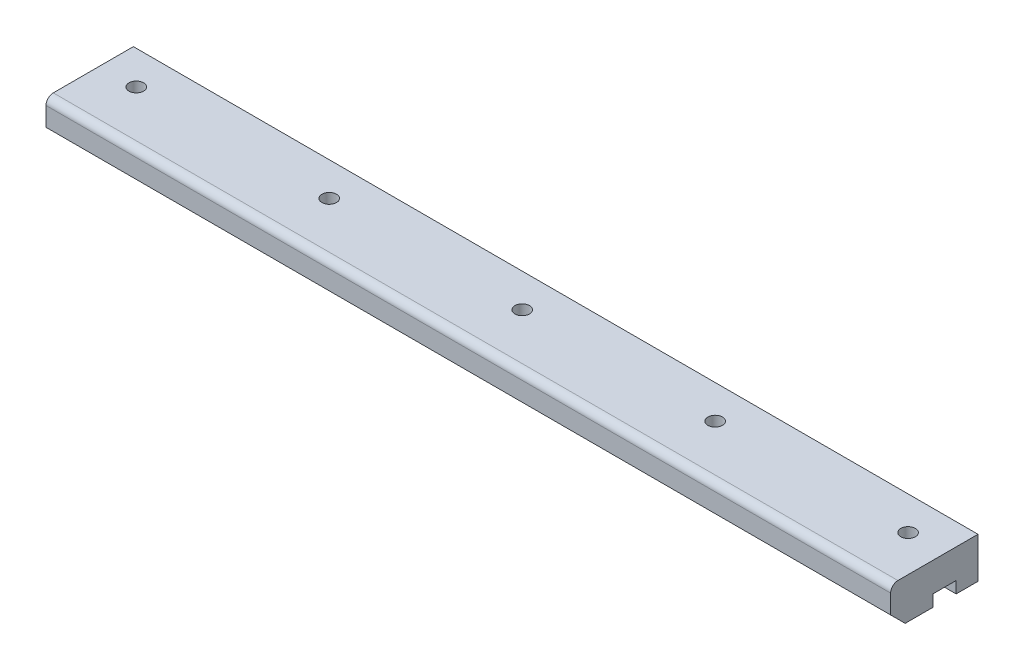
ISO-10303-21;
HEADER;
FILE_DESCRIPTION(('STEP AP214'),'2;1');
FILE_NAME('part.step','',(''),(''),'','','');
FILE_SCHEMA(('AUTOMOTIVE_DESIGN { 1 0 10303 214 1 1 1 1 }'));
ENDSEC;
DATA;
#1=APPLICATION_CONTEXT('core data for automotive mechanical design processes');
#2=APPLICATION_PROTOCOL_DEFINITION('international standard','automotive_design',2000,#1);
#3=PRODUCT_CONTEXT('',#1,'mechanical');
#4=PRODUCT('Part','Part','',(#3));
#5=PRODUCT_RELATED_PRODUCT_CATEGORY('part','',(#4));
#6=PRODUCT_DEFINITION_FORMATION('','',#4);
#7=PRODUCT_DEFINITION_CONTEXT('part definition',#1,'design');
#8=PRODUCT_DEFINITION('design','',#6,#7);
#9=PRODUCT_DEFINITION_SHAPE('','',#8);
#10=(LENGTH_UNIT() NAMED_UNIT(*) SI_UNIT(.MILLI.,.METRE.));
#11=(NAMED_UNIT(*) PLANE_ANGLE_UNIT() SI_UNIT($,.RADIAN.));
#12=(NAMED_UNIT(*) SI_UNIT($,.STERADIAN.) SOLID_ANGLE_UNIT());
#13=UNCERTAINTY_MEASURE_WITH_UNIT(LENGTH_MEASURE(1.E-05),#10,'distance_accuracy_value','');
#14=(GEOMETRIC_REPRESENTATION_CONTEXT(3) GLOBAL_UNCERTAINTY_ASSIGNED_CONTEXT((#13)) GLOBAL_UNIT_ASSIGNED_CONTEXT((#10,
#11,#12)) REPRESENTATION_CONTEXT('',''));
#15=CARTESIAN_POINT('',(0.,0.,0.));
#16=DIRECTION('',(0.,0.,1.));
#17=DIRECTION('',(1.,0.,0.));
#18=AXIS2_PLACEMENT_3D('',#15,#16,#17);
#19=CARTESIAN_POINT('',(580.,28.,-30.));
#20=DIRECTION('',(0.,0.,1.));
#21=DIRECTION('',(1.,0.,0.));
#22=AXIS2_PLACEMENT_3D('',#19,#20,#21);
#23=PLANE('',#22);
#24=DIRECTION('',(0.,1.,0.));
#25=VECTOR('',#24,1.);
#26=CARTESIAN_POINT('',(0.,28.,-30.));
#27=LINE('',#26,#25);
#28=CARTESIAN_POINT('',(0.,0.,-30.));
#29=VERTEX_POINT('',#28);
#30=CARTESIAN_POINT('',(0.,28.,-30.));
#31=VERTEX_POINT('',#30);
#32=EDGE_CURVE('E149',#29,#31,#27,.T.);
#33=ORIENTED_EDGE('',*,*,#32,.T.);
#34=DIRECTION('',(-1.,0.,0.));
#35=VECTOR('',#34,1.);
#36=CARTESIAN_POINT('',(580.,28.,-30.));
#37=LINE('',#36,#35);
#38=CARTESIAN_POINT('',(580.,28.,-30.));
#39=VERTEX_POINT('',#38);
#40=EDGE_CURVE('E11',#39,#31,#37,.T.);
#41=ORIENTED_EDGE('',*,*,#40,.F.);
#42=DIRECTION('',(0.,1.,0.));
#43=VECTOR('',#42,1.);
#44=CARTESIAN_POINT('',(580.,28.,-30.));
#45=LINE('',#44,#43);
#46=CARTESIAN_POINT('',(580.,0.,-30.));
#47=VERTEX_POINT('',#46);
#48=EDGE_CURVE('E170',#47,#39,#45,.T.);
#49=ORIENTED_EDGE('',*,*,#48,.F.);
#50=DIRECTION('',(-1.,0.,0.));
#51=VECTOR('',#50,1.);
#52=CARTESIAN_POINT('',(580.,0.,-30.));
#53=LINE('',#52,#51);
#54=EDGE_CURVE('E144',#47,#29,#53,.T.);
#55=ORIENTED_EDGE('',*,*,#54,.T.);
#56=EDGE_LOOP('',(#33,#41,#49,#55));
#57=FACE_BOUND('',#56,.T.);
#58=ADVANCED_FACE('F39',(#57),#23,.F.);
#59=CARTESIAN_POINT('',(580.,28.,25.));
#60=DIRECTION('',(0.,-1.,0.));
#61=DIRECTION('',(0.,0.,-1.));
#62=AXIS2_PLACEMENT_3D('',#59,#60,#61);
#63=PLANE('',#62);
#64=CARTESIAN_POINT('',(25.,28.,-7.));
#65=DIRECTION('',(0.,1.,0.));
#66=DIRECTION('',(0.,0.,1.));
#67=AXIS2_PLACEMENT_3D('',#64,#65,#66);
#68=CIRCLE('',#67,5.);
#69=CARTESIAN_POINT('',(25.,28.,-1.99999999999999));
#70=VERTEX_POINT('',#69);
#71=EDGE_CURVE('E188',#70,#70,#68,.T.);
#72=ORIENTED_EDGE('',*,*,#71,.F.);
#73=EDGE_LOOP('',(#72));
#74=FACE_BOUND('',#73,.T.);
#75=CARTESIAN_POINT('',(157.5,28.,-7.));
#76=DIRECTION('',(0.,1.,0.));
#77=DIRECTION('',(0.,0.,1.));
#78=AXIS2_PLACEMENT_3D('',#75,#76,#77);
#79=CIRCLE('',#78,4.99999999999999);
#80=CARTESIAN_POINT('',(157.5,28.,-2.00000000000001));
#81=VERTEX_POINT('',#80);
#82=EDGE_CURVE('E306',#81,#81,#79,.T.);
#83=ORIENTED_EDGE('',*,*,#82,.F.);
#84=EDGE_LOOP('',(#83));
#85=FACE_BOUND('',#84,.T.);
#86=CARTESIAN_POINT('',(290.,28.,-7.));
#87=DIRECTION('',(0.,1.,0.));
#88=DIRECTION('',(0.,0.,1.));
#89=AXIS2_PLACEMENT_3D('',#86,#87,#88);
#90=CIRCLE('',#89,4.99999999999999);
#91=CARTESIAN_POINT('',(290.,28.,-2.00000000000001));
#92=VERTEX_POINT('',#91);
#93=EDGE_CURVE('E300',#92,#92,#90,.T.);
#94=ORIENTED_EDGE('',*,*,#93,.F.);
#95=EDGE_LOOP('',(#94));
#96=FACE_BOUND('',#95,.T.);
#97=CARTESIAN_POINT('',(422.5,28.,-7.));
#98=DIRECTION('',(0.,1.,0.));
#99=DIRECTION('',(0.,0.,1.));
#100=AXIS2_PLACEMENT_3D('',#97,#98,#99);
#101=CIRCLE('',#100,4.99999999999999);
#102=CARTESIAN_POINT('',(422.5,28.,-2.00000000000001));
#103=VERTEX_POINT('',#102);
#104=EDGE_CURVE('E310',#103,#103,#101,.T.);
#105=ORIENTED_EDGE('',*,*,#104,.F.);
#106=EDGE_LOOP('',(#105));
#107=FACE_BOUND('',#106,.T.);
#108=CARTESIAN_POINT('',(555.,28.,-7.));
#109=DIRECTION('',(0.,1.,0.));
#110=DIRECTION('',(0.,0.,1.));
#111=AXIS2_PLACEMENT_3D('',#108,#109,#110);
#112=CIRCLE('',#111,5.00000000000004);
#113=CARTESIAN_POINT('',(555.,28.,-1.99999999999995));
#114=VERTEX_POINT('',#113);
#115=EDGE_CURVE('E314',#114,#114,#112,.T.);
#116=ORIENTED_EDGE('',*,*,#115,.F.);
#117=EDGE_LOOP('',(#116));
#118=FACE_BOUND('',#117,.T.);
#119=DIRECTION('',(0.,0.,1.));
#120=VECTOR('',#119,1.);
#121=CARTESIAN_POINT('',(0.,28.,25.));
#122=LINE('',#121,#120);
#123=CARTESIAN_POINT('',(0.,28.,25.));
#124=VERTEX_POINT('',#123);
#125=EDGE_CURVE('E155',#31,#124,#122,.T.);
#126=ORIENTED_EDGE('',*,*,#125,.T.);
#127=DIRECTION('',(-1.,0.,0.));
#128=VECTOR('',#127,1.);
#129=CARTESIAN_POINT('',(580.,28.,25.));
#130=LINE('',#129,#128);
#131=CARTESIAN_POINT('',(580.,28.,25.));
#132=VERTEX_POINT('',#131);
#133=EDGE_CURVE('E48',#132,#124,#130,.T.);
#134=ORIENTED_EDGE('',*,*,#133,.F.);
#135=DIRECTION('',(0.,0.,1.));
#136=VECTOR('',#135,1.);
#137=CARTESIAN_POINT('',(580.,28.,25.));
#138=LINE('',#137,#136);
#139=EDGE_CURVE('E106',#39,#132,#138,.T.);
#140=ORIENTED_EDGE('',*,*,#139,.F.);
#141=ORIENTED_EDGE('',*,*,#40,.T.);
#142=EDGE_LOOP('',(#126,#134,#140,#141));
#143=FACE_BOUND('',#142,.T.);
#144=ADVANCED_FACE('F214',(#74,#85,#96,#107,#118,#143),#63,.F.);
#145=CARTESIAN_POINT('',(580.,23.,25.));
#146=DIRECTION('',(-1.,0.,0.));
#147=DIRECTION('',(0.,0.,1.));
#148=AXIS2_PLACEMENT_3D('',#145,#146,#147);
#149=CYLINDRICAL_SURFACE('',#148,5.);
#150=CARTESIAN_POINT('',(0.,23.,25.));
#151=DIRECTION('',(1.,0.,0.));
#152=DIRECTION('',(0.,0.,-1.));
#153=AXIS2_PLACEMENT_3D('',#150,#151,#152);
#154=CIRCLE('',#153,5.);
#155=CARTESIAN_POINT('',(0.,23.,30.));
#156=VERTEX_POINT('',#155);
#157=EDGE_CURVE('E152',#124,#156,#154,.T.);
#158=ORIENTED_EDGE('',*,*,#157,.T.);
#159=DIRECTION('',(-1.,0.,0.));
#160=VECTOR('',#159,1.);
#161=CARTESIAN_POINT('',(580.,23.,30.));
#162=LINE('',#161,#160);
#163=CARTESIAN_POINT('',(580.,23.,30.));
#164=VERTEX_POINT('',#163);
#165=EDGE_CURVE('E176',#164,#156,#162,.T.);
#166=ORIENTED_EDGE('',*,*,#165,.F.);
#167=CARTESIAN_POINT('',(580.,23.,25.));
#168=DIRECTION('',(1.,0.,0.));
#169=DIRECTION('',(0.,0.,-1.));
#170=AXIS2_PLACEMENT_3D('',#167,#168,#169);
#171=CIRCLE('',#170,5.);
#172=EDGE_CURVE('E233',#132,#164,#171,.T.);
#173=ORIENTED_EDGE('',*,*,#172,.F.);
#174=ORIENTED_EDGE('',*,*,#133,.T.);
#175=EDGE_LOOP('',(#158,#166,#173,#174));
#176=FACE_BOUND('',#175,.T.);
#177=ADVANCED_FACE('F222',(#176),#149,.T.);
#178=CARTESIAN_POINT('',(580.,10.,30.));
#179=DIRECTION('',(0.,0.,-1.));
#180=DIRECTION('',(-1.,0.,0.));
#181=AXIS2_PLACEMENT_3D('',#178,#179,#180);
#182=PLANE('',#181);
#183=DIRECTION('',(0.,-1.,0.));
#184=VECTOR('',#183,1.);
#185=CARTESIAN_POINT('',(0.,10.,30.));
#186=LINE('',#185,#184);
#187=CARTESIAN_POINT('',(0.,10.,30.));
#188=VERTEX_POINT('',#187);
#189=EDGE_CURVE('E156',#156,#188,#186,.T.);
#190=ORIENTED_EDGE('',*,*,#189,.T.);
#191=DIRECTION('',(-1.,0.,0.));
#192=VECTOR('',#191,1.);
#193=CARTESIAN_POINT('',(580.,10.,30.));
#194=LINE('',#193,#192);
#195=CARTESIAN_POINT('',(580.,10.,30.));
#196=VERTEX_POINT('',#195);
#197=EDGE_CURVE('E180',#196,#188,#194,.T.);
#198=ORIENTED_EDGE('',*,*,#197,.F.);
#199=DIRECTION('',(0.,-1.,0.));
#200=VECTOR('',#199,1.);
#201=CARTESIAN_POINT('',(580.,10.,30.));
#202=LINE('',#201,#200);
#203=EDGE_CURVE('E231',#164,#196,#202,.T.);
#204=ORIENTED_EDGE('',*,*,#203,.F.);
#205=ORIENTED_EDGE('',*,*,#165,.T.);
#206=EDGE_LOOP('',(#190,#198,#204,#205));
#207=FACE_BOUND('',#206,.T.);
#208=ADVANCED_FACE('F259',(#207),#182,.F.);
#209=CARTESIAN_POINT('',(580.,0.,20.));
#210=DIRECTION('',(0.,0.707106781186547,-0.707106781186548));
#211=DIRECTION('',(0.,0.707106781186548,0.707106781186547));
#212=AXIS2_PLACEMENT_3D('',#209,#210,#211);
#213=PLANE('',#212);
#214=DIRECTION('',(0.,-0.707106781186548,-0.707106781186547));
#215=VECTOR('',#214,1.);
#216=CARTESIAN_POINT('',(0.,0.,20.));
#217=LINE('',#216,#215);
#218=CARTESIAN_POINT('',(0.,0.,20.));
#219=VERTEX_POINT('',#218);
#220=EDGE_CURVE('E158',#188,#219,#217,.T.);
#221=ORIENTED_EDGE('',*,*,#220,.T.);
#222=DIRECTION('',(-1.,0.,0.));
#223=VECTOR('',#222,1.);
#224=CARTESIAN_POINT('',(580.,0.,20.));
#225=LINE('',#224,#223);
#226=CARTESIAN_POINT('',(580.,0.,20.));
#227=VERTEX_POINT('',#226);
#228=EDGE_CURVE('E173',#227,#219,#225,.T.);
#229=ORIENTED_EDGE('',*,*,#228,.F.);
#230=DIRECTION('',(0.,-0.707106781186548,-0.707106781186547));
#231=VECTOR('',#230,1.);
#232=CARTESIAN_POINT('',(580.,0.,20.));
#233=LINE('',#232,#231);
#234=EDGE_CURVE('E240',#196,#227,#233,.T.);
#235=ORIENTED_EDGE('',*,*,#234,.F.);
#236=ORIENTED_EDGE('',*,*,#197,.T.);
#237=EDGE_LOOP('',(#221,#229,#235,#236));
#238=FACE_BOUND('',#237,.T.);
#239=ADVANCED_FACE('F258',(#238),#213,.F.);
#240=CARTESIAN_POINT('',(580.,0.,1.));
#241=DIRECTION('',(0.,1.,0.));
#242=DIRECTION('',(0.,0.,1.));
#243=AXIS2_PLACEMENT_3D('',#240,#241,#242);
#244=PLANE('',#243);
#245=DIRECTION('',(0.,0.,-1.));
#246=VECTOR('',#245,1.);
#247=CARTESIAN_POINT('',(0.,0.,1.));
#248=LINE('',#247,#246);
#249=CARTESIAN_POINT('',(0.,0.,1.));
#250=VERTEX_POINT('',#249);
#251=EDGE_CURVE('E159',#219,#250,#248,.T.);
#252=ORIENTED_EDGE('',*,*,#251,.T.);
#253=DIRECTION('',(-1.,0.,0.));
#254=VECTOR('',#253,1.);
#255=CARTESIAN_POINT('',(580.,0.,1.));
#256=LINE('',#255,#254);
#257=CARTESIAN_POINT('',(580.,0.,1.));
#258=VERTEX_POINT('',#257);
#259=EDGE_CURVE('E174',#258,#250,#256,.T.);
#260=ORIENTED_EDGE('',*,*,#259,.F.);
#261=DIRECTION('',(0.,0.,-1.));
#262=VECTOR('',#261,1.);
#263=CARTESIAN_POINT('',(580.,0.,1.));
#264=LINE('',#263,#262);
#265=EDGE_CURVE('E245',#227,#258,#264,.T.);
#266=ORIENTED_EDGE('',*,*,#265,.F.);
#267=ORIENTED_EDGE('',*,*,#228,.T.);
#268=EDGE_LOOP('',(#252,#260,#266,#267));
#269=FACE_BOUND('',#268,.T.);
#270=ADVANCED_FACE('F249',(#269),#244,.F.);
#271=CARTESIAN_POINT('',(580.,8.,1.));
#272=DIRECTION('',(0.,0.,1.));
#273=DIRECTION('',(1.,0.,0.));
#274=AXIS2_PLACEMENT_3D('',#271,#272,#273);
#275=PLANE('',#274);
#276=DIRECTION('',(0.,1.,0.));
#277=VECTOR('',#276,1.);
#278=CARTESIAN_POINT('',(0.,8.,1.));
#279=LINE('',#278,#277);
#280=CARTESIAN_POINT('',(0.,8.,1.));
#281=VERTEX_POINT('',#280);
#282=EDGE_CURVE('E165',#250,#281,#279,.T.);
#283=ORIENTED_EDGE('',*,*,#282,.T.);
#284=DIRECTION('',(-1.,0.,0.));
#285=VECTOR('',#284,1.);
#286=CARTESIAN_POINT('',(580.,8.,1.));
#287=LINE('',#286,#285);
#288=CARTESIAN_POINT('',(580.,8.,1.));
#289=VERTEX_POINT('',#288);
#290=EDGE_CURVE('E136',#289,#281,#287,.T.);
#291=ORIENTED_EDGE('',*,*,#290,.F.);
#292=DIRECTION('',(0.,1.,0.));
#293=VECTOR('',#292,1.);
#294=CARTESIAN_POINT('',(580.,8.,1.));
#295=LINE('',#294,#293);
#296=EDGE_CURVE('E134',#258,#289,#295,.T.);
#297=ORIENTED_EDGE('',*,*,#296,.F.);
#298=ORIENTED_EDGE('',*,*,#259,.T.);
#299=EDGE_LOOP('',(#283,#291,#297,#298));
#300=FACE_BOUND('',#299,.T.);
#301=ADVANCED_FACE('F251',(#300),#275,.F.);
#302=CARTESIAN_POINT('',(580.,8.,-15.));
#303=DIRECTION('',(0.,1.,0.));
#304=DIRECTION('',(0.,0.,1.));
#305=AXIS2_PLACEMENT_3D('',#302,#303,#304);
#306=PLANE('',#305);
#307=CARTESIAN_POINT('',(25.,8.00000000000001,-7.));
#308=DIRECTION('',(0.,1.,0.));
#309=DIRECTION('',(0.,0.,1.));
#310=AXIS2_PLACEMENT_3D('',#307,#308,#309);
#311=CIRCLE('',#310,5.);
#312=CARTESIAN_POINT('',(25.,8.00000000000001,-1.99999999999999));
#313=VERTEX_POINT('',#312);
#314=EDGE_CURVE('E45',#313,#313,#311,.T.);
#315=ORIENTED_EDGE('',*,*,#314,.T.);
#316=EDGE_LOOP('',(#315));
#317=FACE_BOUND('',#316,.T.);
#318=CARTESIAN_POINT('',(157.5,8.00000000000001,-7.));
#319=DIRECTION('',(0.,1.,0.));
#320=DIRECTION('',(0.,0.,1.));
#321=AXIS2_PLACEMENT_3D('',#318,#319,#320);
#322=CIRCLE('',#321,4.99999999999999);
#323=CARTESIAN_POINT('',(157.5,8.00000000000001,-2.00000000000001));
#324=VERTEX_POINT('',#323);
#325=EDGE_CURVE('E194',#324,#324,#322,.T.);
#326=ORIENTED_EDGE('',*,*,#325,.T.);
#327=EDGE_LOOP('',(#326));
#328=FACE_BOUND('',#327,.T.);
#329=CARTESIAN_POINT('',(290.,8.00000000000001,-7.));
#330=DIRECTION('',(0.,1.,0.));
#331=DIRECTION('',(0.,0.,1.));
#332=AXIS2_PLACEMENT_3D('',#329,#330,#331);
#333=CIRCLE('',#332,4.99999999999999);
#334=CARTESIAN_POINT('',(290.,8.00000000000001,-2.00000000000001));
#335=VERTEX_POINT('',#334);
#336=EDGE_CURVE('E195',#335,#335,#333,.T.);
#337=ORIENTED_EDGE('',*,*,#336,.T.);
#338=EDGE_LOOP('',(#337));
#339=FACE_BOUND('',#338,.T.);
#340=CARTESIAN_POINT('',(422.5,8.00000000000001,-7.));
#341=DIRECTION('',(0.,1.,0.));
#342=DIRECTION('',(0.,0.,1.));
#343=AXIS2_PLACEMENT_3D('',#340,#341,#342);
#344=CIRCLE('',#343,4.99999999999999);
#345=CARTESIAN_POINT('',(422.5,8.00000000000001,-2.00000000000001));
#346=VERTEX_POINT('',#345);
#347=EDGE_CURVE('E190',#346,#346,#344,.T.);
#348=ORIENTED_EDGE('',*,*,#347,.T.);
#349=EDGE_LOOP('',(#348));
#350=FACE_BOUND('',#349,.T.);
#351=CARTESIAN_POINT('',(555.,8.00000000000001,-7.));
#352=DIRECTION('',(0.,1.,0.));
#353=DIRECTION('',(0.,0.,1.));
#354=AXIS2_PLACEMENT_3D('',#351,#352,#353);
#355=CIRCLE('',#354,5.00000000000004);
#356=CARTESIAN_POINT('',(555.,8.00000000000001,-1.99999999999995));
#357=VERTEX_POINT('',#356);
#358=EDGE_CURVE('E183',#357,#357,#355,.T.);
#359=ORIENTED_EDGE('',*,*,#358,.T.);
#360=EDGE_LOOP('',(#359));
#361=FACE_BOUND('',#360,.T.);
#362=DIRECTION('',(0.,0.,-1.));
#363=VECTOR('',#362,1.);
#364=CARTESIAN_POINT('',(0.,8.,-15.));
#365=LINE('',#364,#363);
#366=CARTESIAN_POINT('',(0.,8.,-15.));
#367=VERTEX_POINT('',#366);
#368=EDGE_CURVE('E139',#281,#367,#365,.T.);
#369=ORIENTED_EDGE('',*,*,#368,.T.);
#370=DIRECTION('',(-1.,0.,0.));
#371=VECTOR('',#370,1.);
#372=CARTESIAN_POINT('',(580.,8.,-15.));
#373=LINE('',#372,#371);
#374=CARTESIAN_POINT('',(580.,8.,-15.));
#375=VERTEX_POINT('',#374);
#376=EDGE_CURVE('E137',#375,#367,#373,.T.);
#377=ORIENTED_EDGE('',*,*,#376,.F.);
#378=DIRECTION('',(0.,0.,-1.));
#379=VECTOR('',#378,1.);
#380=CARTESIAN_POINT('',(580.,8.,-15.));
#381=LINE('',#380,#379);
#382=EDGE_CURVE('E121',#289,#375,#381,.T.);
#383=ORIENTED_EDGE('',*,*,#382,.F.);
#384=ORIENTED_EDGE('',*,*,#290,.T.);
#385=EDGE_LOOP('',(#369,#377,#383,#384));
#386=FACE_BOUND('',#385,.T.);
#387=ADVANCED_FACE('F140',(#317,#328,#339,#350,#361,#386),#306,.F.);
#388=CARTESIAN_POINT('',(580.,0.,-15.));
#389=DIRECTION('',(0.,0.,-1.));
#390=DIRECTION('',(-1.,0.,0.));
#391=AXIS2_PLACEMENT_3D('',#388,#389,#390);
#392=PLANE('',#391);
#393=DIRECTION('',(0.,-1.,0.));
#394=VECTOR('',#393,1.);
#395=CARTESIAN_POINT('',(0.,0.,-15.));
#396=LINE('',#395,#394);
#397=CARTESIAN_POINT('',(0.,0.,-15.));
#398=VERTEX_POINT('',#397);
#399=EDGE_CURVE('E95',#367,#398,#396,.T.);
#400=ORIENTED_EDGE('',*,*,#399,.T.);
#401=DIRECTION('',(-1.,0.,0.));
#402=VECTOR('',#401,1.);
#403=CARTESIAN_POINT('',(580.,0.,-15.));
#404=LINE('',#403,#402);
#405=CARTESIAN_POINT('',(580.,0.,-15.));
#406=VERTEX_POINT('',#405);
#407=EDGE_CURVE('E143',#406,#398,#404,.T.);
#408=ORIENTED_EDGE('',*,*,#407,.F.);
#409=DIRECTION('',(0.,-1.,0.));
#410=VECTOR('',#409,1.);
#411=CARTESIAN_POINT('',(580.,0.,-15.));
#412=LINE('',#411,#410);
#413=EDGE_CURVE('E129',#375,#406,#412,.T.);
#414=ORIENTED_EDGE('',*,*,#413,.F.);
#415=ORIENTED_EDGE('',*,*,#376,.T.);
#416=EDGE_LOOP('',(#400,#408,#414,#415));
#417=FACE_BOUND('',#416,.T.);
#418=ADVANCED_FACE('F141',(#417),#392,.F.);
#419=CARTESIAN_POINT('',(580.,0.,-30.));
#420=DIRECTION('',(0.,1.,0.));
#421=DIRECTION('',(0.,0.,1.));
#422=AXIS2_PLACEMENT_3D('',#419,#420,#421);
#423=PLANE('',#422);
#424=DIRECTION('',(0.,0.,-1.));
#425=VECTOR('',#424,1.);
#426=CARTESIAN_POINT('',(0.,0.,-30.));
#427=LINE('',#426,#425);
#428=EDGE_CURVE('E98',#398,#29,#427,.T.);
#429=ORIENTED_EDGE('',*,*,#428,.T.);
#430=ORIENTED_EDGE('',*,*,#54,.F.);
#431=DIRECTION('',(0.,0.,-1.));
#432=VECTOR('',#431,1.);
#433=CARTESIAN_POINT('',(580.,0.,-30.));
#434=LINE('',#433,#432);
#435=EDGE_CURVE('E60',#406,#47,#434,.T.);
#436=ORIENTED_EDGE('',*,*,#435,.F.);
#437=ORIENTED_EDGE('',*,*,#407,.T.);
#438=EDGE_LOOP('',(#429,#430,#436,#437));
#439=FACE_BOUND('',#438,.T.);
#440=ADVANCED_FACE('F277',(#439),#423,.F.);
#441=CARTESIAN_POINT('',(580.,23.,25.));
#442=DIRECTION('',(1.,0.,0.));
#443=DIRECTION('',(0.,0.,-1.));
#444=AXIS2_PLACEMENT_3D('',#441,#442,#443);
#445=PLANE('',#444);
#446=ORIENTED_EDGE('',*,*,#48,.T.);
#447=ORIENTED_EDGE('',*,*,#139,.T.);
#448=ORIENTED_EDGE('',*,*,#172,.T.);
#449=ORIENTED_EDGE('',*,*,#203,.T.);
#450=ORIENTED_EDGE('',*,*,#234,.T.);
#451=ORIENTED_EDGE('',*,*,#265,.T.);
#452=ORIENTED_EDGE('',*,*,#296,.T.);
#453=ORIENTED_EDGE('',*,*,#382,.T.);
#454=ORIENTED_EDGE('',*,*,#413,.T.);
#455=ORIENTED_EDGE('',*,*,#435,.T.);
#456=EDGE_LOOP('',(#446,#447,#448,#449,#450,#451,#452,#453,#454,#455));
#457=FACE_BOUND('',#456,.T.);
#458=ADVANCED_FACE('F130',(#457),#445,.T.);
#459=CARTESIAN_POINT('',(0.,23.,25.));
#460=DIRECTION('',(1.,0.,0.));
#461=DIRECTION('',(0.,0.,-1.));
#462=AXIS2_PLACEMENT_3D('',#459,#460,#461);
#463=PLANE('',#462);
#464=ORIENTED_EDGE('',*,*,#32,.F.);
#465=ORIENTED_EDGE('',*,*,#428,.F.);
#466=ORIENTED_EDGE('',*,*,#399,.F.);
#467=ORIENTED_EDGE('',*,*,#368,.F.);
#468=ORIENTED_EDGE('',*,*,#282,.F.);
#469=ORIENTED_EDGE('',*,*,#251,.F.);
#470=ORIENTED_EDGE('',*,*,#220,.F.);
#471=ORIENTED_EDGE('',*,*,#189,.F.);
#472=ORIENTED_EDGE('',*,*,#157,.F.);
#473=ORIENTED_EDGE('',*,*,#125,.F.);
#474=EDGE_LOOP('',(#464,#465,#466,#467,#468,#469,#470,#471,#472,#473));
#475=FACE_BOUND('',#474,.T.);
#476=ADVANCED_FACE('F226',(#475),#463,.F.);
#477=CARTESIAN_POINT('',(555.,-552.,-7.));
#478=DIRECTION('',(0.,1.,0.));
#479=DIRECTION('',(0.,0.,1.));
#480=AXIS2_PLACEMENT_3D('',#477,#478,#479);
#481=CYLINDRICAL_SURFACE('',#480,5.00000000000004);
#482=ORIENTED_EDGE('',*,*,#115,.T.);
#483=EDGE_LOOP('',(#482));
#484=FACE_BOUND('',#483,.T.);
#485=ORIENTED_EDGE('',*,*,#358,.F.);
#486=EDGE_LOOP('',(#485));
#487=FACE_BOUND('',#486,.T.);
#488=ADVANCED_FACE('F284',(#484,#487),#481,.F.);
#489=CARTESIAN_POINT('',(422.5,-552.,-7.));
#490=DIRECTION('',(0.,1.,0.));
#491=DIRECTION('',(0.,0.,1.));
#492=AXIS2_PLACEMENT_3D('',#489,#490,#491);
#493=CYLINDRICAL_SURFACE('',#492,4.99999999999999);
#494=ORIENTED_EDGE('',*,*,#104,.T.);
#495=EDGE_LOOP('',(#494));
#496=FACE_BOUND('',#495,.T.);
#497=ORIENTED_EDGE('',*,*,#347,.F.);
#498=EDGE_LOOP('',(#497));
#499=FACE_BOUND('',#498,.T.);
#500=ADVANCED_FACE('F287',(#496,#499),#493,.F.);
#501=CARTESIAN_POINT('',(290.,-552.,-7.));
#502=DIRECTION('',(0.,1.,0.));
#503=DIRECTION('',(0.,0.,1.));
#504=AXIS2_PLACEMENT_3D('',#501,#502,#503);
#505=CYLINDRICAL_SURFACE('',#504,4.99999999999999);
#506=ORIENTED_EDGE('',*,*,#93,.T.);
#507=EDGE_LOOP('',(#506));
#508=FACE_BOUND('',#507,.T.);
#509=ORIENTED_EDGE('',*,*,#336,.F.);
#510=EDGE_LOOP('',(#509));
#511=FACE_BOUND('',#510,.T.);
#512=ADVANCED_FACE('F209',(#508,#511),#505,.F.);
#513=CARTESIAN_POINT('',(157.5,-552.,-7.));
#514=DIRECTION('',(0.,1.,0.));
#515=DIRECTION('',(0.,0.,1.));
#516=AXIS2_PLACEMENT_3D('',#513,#514,#515);
#517=CYLINDRICAL_SURFACE('',#516,4.99999999999999);
#518=ORIENTED_EDGE('',*,*,#82,.T.);
#519=EDGE_LOOP('',(#518));
#520=FACE_BOUND('',#519,.T.);
#521=ORIENTED_EDGE('',*,*,#325,.F.);
#522=EDGE_LOOP('',(#521));
#523=FACE_BOUND('',#522,.T.);
#524=ADVANCED_FACE('F204',(#520,#523),#517,.F.);
#525=CARTESIAN_POINT('',(25.,-552.,-7.));
#526=DIRECTION('',(0.,1.,0.));
#527=DIRECTION('',(0.,0.,1.));
#528=AXIS2_PLACEMENT_3D('',#525,#526,#527);
#529=CYLINDRICAL_SURFACE('',#528,5.);
#530=ORIENTED_EDGE('',*,*,#71,.T.);
#531=EDGE_LOOP('',(#530));
#532=FACE_BOUND('',#531,.T.);
#533=ORIENTED_EDGE('',*,*,#314,.F.);
#534=EDGE_LOOP('',(#533));
#535=FACE_BOUND('',#534,.T.);
#536=ADVANCED_FACE('F205',(#532,#535),#529,.F.);
#537=CLOSED_SHELL('',(#58,#144,#177,#208,#239,#270,#301,#387,#418,#440,#458,#476,#488,#500,#512,
#524,#536));
#538=MANIFOLD_SOLID_BREP('B2',#537);
#539=ADVANCED_BREP_SHAPE_REPRESENTATION('',(#18,#538),#14);
#540=SHAPE_DEFINITION_REPRESENTATION(#9,#539);
ENDSEC;
END-ISO-10303-21;
